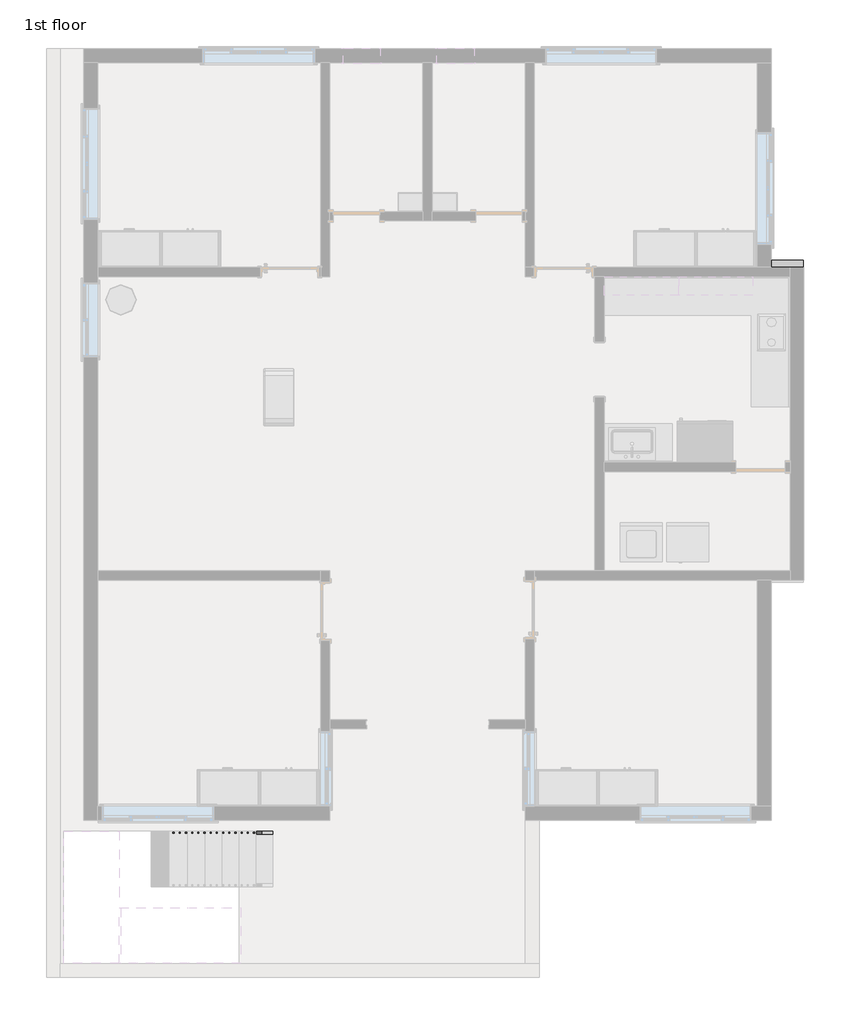
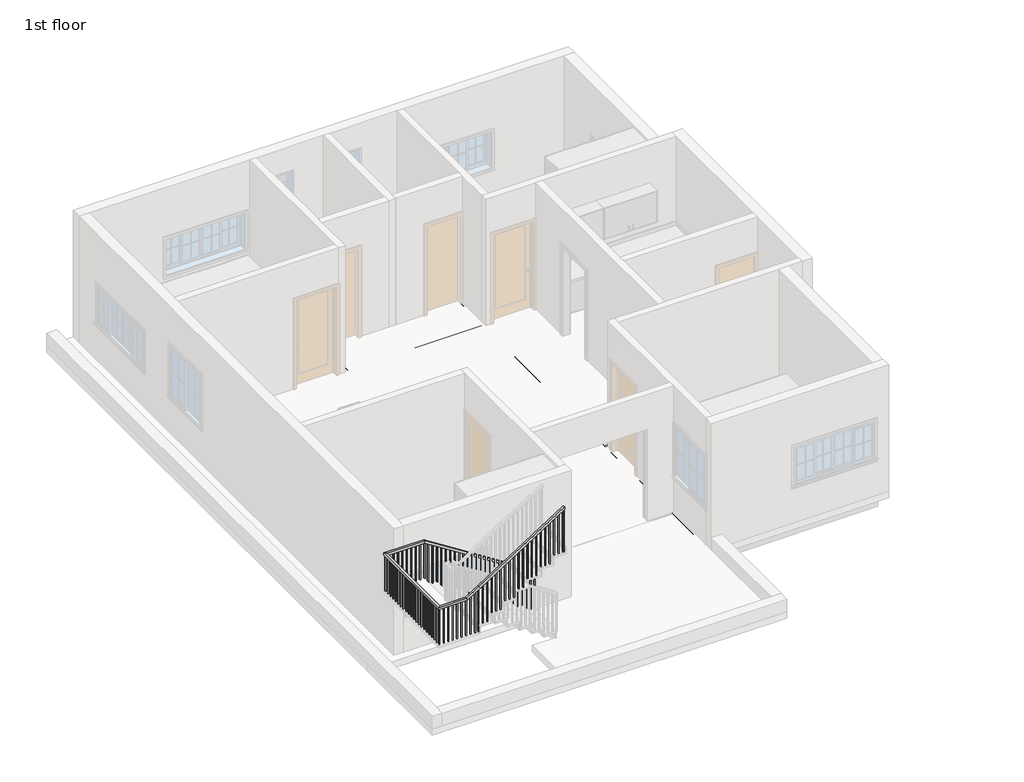
# One storey, part 2 of 4: 6 beams, 1 railing.
"""IFC4 building model written with IfcOpenShell, lengths in millimetres."""

from ifc_helpers import new_model, si_unit, frame, origin, place, context, project, spatial, polyline, outline, extrude, faceted_brep, element, save

model = new_model("IFC4")

# Units and contexts
model_context = context("Model", 3, world=origin())
ifc_project = project(units=[si_unit("LENGTHUNIT", "METRE", prefix="MILLI")], contexts=[model_context])

# Site, building, storey
site = spatial("IfcSite", under=ifc_project)
building = spatial("IfcBuilding", under=site)
storey = spatial("IfcBuildingStorey", under=building, Name="1st floor", Elevation=3810.0)

# Beams
placement = place(None, origin())
element("IfcBeam", 1, ObjectType="Concrete-Rectangular Beam", at=placement, inside=storey, context=model_context, shape_type="Brep", body=[
    faceted_brep([(-12413.6124084, 10142.6961804, 3810.0), (-12413.6124084, 9914.0961804, 3810.0), (-8794.1124084, 9914.0961804, 3810.0), (-8565.5124084, 9914.0961804, 3810.0), (-7117.7124084, 9914.0961804, 3810.0), (-6889.1124084, 9914.0961804, 3810.0), (-5441.3124084, 9914.0961804, 3810.0), (-5212.7124084, 9914.0961804, 3810.0), (-1593.2124084, 9914.0961804, 3810.0), (-1593.2124084, 10142.6961804, 3810.0), (-5174.6124084, 10142.6961804, 3810.0), (-5174.6124084, 9952.1961804, 3810.0), (-5479.4124084, 9952.1961804, 3810.0), (-5479.4124084, 10142.6961804, 3810.0), (-8451.2124084, 10142.6961804, 3810.0), (-8451.2124084, 9952.1961804, 3810.0), (-8756.0124084, 9952.1961804, 3810.0), (-8756.0124084, 10142.6961804, 3810.0), (-12413.6124084, 9914.0961804, 3505.2), (-8794.1124084, 9914.0961804, 3505.2), (-8565.5124084, 9914.0961804, 3505.2), (-7117.7124084, 9914.0961804, 3505.2), (-6889.1124084, 9914.0961804, 3505.2), (-5441.3124084, 9914.0961804, 3505.2), (-5212.7124084, 9914.0961804, 3505.2), (-1593.2124084, 9914.0961804, 3505.2), (-12413.6124084, 10142.6961804, 3505.2), (-8756.0124084, 10142.6961804, 3505.2), (-8756.0124084, 9952.1961804, 3505.2), (-8451.2124084, 9952.1961804, 3505.2), (-8451.2124084, 10142.6961804, 3505.2), (-5479.4124084, 10142.6961804, 3505.2), (-5479.4124084, 9952.1961804, 3505.2), (-5174.6124084, 9952.1961804, 3505.2), (-5174.6124084, 10142.6961804, 3505.2), (-1593.2124084, 10142.6961804, 3505.2)], [[[0, 1, 2, 3, 4, 5, 6, 7, 8, 9, 10, 11, 12, 13, 14, 15, 16, 17]], [[1, 18, 19, 20, 21, 22, 23, 24, 25, 8, 7, 6, 5, 4, 3, 2]], [[18, 26, 27, 28, 29, 30, 31, 32, 33, 34, 35, 25, 24, 23, 22, 21, 20, 19]], [[26, 0, 17, 27]], [[1, 0, 26, 18]], [[9, 8, 25, 35]], [[29, 15, 14, 30]], [[15, 29, 28, 16]], [[16, 28, 27, 17]], [[9, 35, 34, 10]], [[33, 11, 10, 34]], [[11, 33, 32, 12]], [[12, 32, 31, 13]], [[30, 14, 13, 31]]]),
])
element("IfcBeam", 2, ObjectType="Concrete-Rectangular Beam", at=placement, inside=storey, context=model_context, shape_type="SweptSolid", body=[
    extrude(outline(polyline([(-1593.2124084, 9875.9961804), (-1364.6124084, 9875.9961804), (-1364.6124084, 6751.7961804), (-1593.2124084, 6751.7961804), (-1593.2124084, 9875.9961804)])), frame((0.0, 0.0, 3505.2), z_axis=(0.0, 0.0, 1.0), x_axis=(1.0, 0.0, 0.0)), (0.0, 0.0, 1.0), 304.8),
])
element("IfcBeam", 3, ObjectType="Concrete-Rectangular Beam", at=placement, inside=storey, context=model_context, shape_type="Brep", body=[
    faceted_brep([(-843.9124084, 6713.6961804, 3810.0), (-843.9124084, 6485.0961804, 3810.0), (-843.9124084, 6485.0961804, 3505.2), (-843.9124084, 6713.6961804, 3505.2), (-1364.6124084, 6713.6961804, 3810.0), (-1364.6124084, 6485.0961804, 3810.0), (-1364.6124084, 6485.0961804, 3505.2), (-1364.6124084, 6713.6961804, 3505.2)], [[[0, 1, 2, 3]], [[1, 0, 4, 5]], [[2, 1, 5, 6]], [[3, 2, 6, 7]], [[0, 3, 7, 4]], [[5, 4, 7, 6]]]),
    faceted_brep([(-12413.6124084, 6485.0961804, 3810.0), (-12413.6124084, 6713.6961804, 3810.0), (-12413.6124084, 6713.6961804, 3505.2), (-12413.6124084, 6485.0961804, 3505.2), (-8756.0124084, 6713.6961804, 3810.0), (-8756.0124084, 6485.0961804, 3810.0), (-8756.0124084, 6485.0961804, 3505.2), (-8756.0124084, 6713.6961804, 3505.2), (-8794.1124084, 6485.0961804, 3810.0), (-8794.1124084, 6713.6961804, 3810.0), (-8794.1124084, 6485.0961804, 3505.2), (-8794.1124084, 6713.6961804, 3505.2)], [[[0, 1, 2, 3]], [[4, 5, 6, 7]], [[1, 0, 8, 5, 4, 9]], [[0, 3, 10, 6, 5, 8]], [[3, 2, 11, 7, 6, 10]], [[2, 1, 9, 4, 7, 11]]]),
    faceted_brep([(-1593.2124084, 6713.6961804, 3810.0), (-1593.2124084, 6485.0961804, 3810.0), (-1593.2124084, 6485.0961804, 3505.2), (-1593.2124084, 6713.6961804, 3505.2), (-5212.7124084, 6713.6961804, 3810.0), (-5250.8124084, 6713.6961804, 3810.0), (-5250.8124084, 6485.0961804, 3810.0), (-5212.7124084, 6485.0961804, 3810.0), (-5250.8124084, 6485.0961804, 3505.2), (-5212.7124084, 6485.0961804, 3505.2), (-5250.8124084, 6713.6961804, 3505.2), (-5212.7124084, 6713.6961804, 3505.2)], [[[0, 1, 2, 3]], [[1, 0, 4, 5, 6, 7]], [[2, 1, 7, 6, 8, 9]], [[3, 2, 9, 8, 10, 11]], [[0, 3, 11, 10, 5, 4]], [[6, 5, 10, 8]]]),
    faceted_brep([(-8527.4124084, 6485.0961804, 3810.0), (-8527.4124084, 6713.6961804, 3810.0), (-8527.4124084, 6713.6961804, 3505.2), (-8527.4124084, 6485.0961804, 3505.2), (-5479.4124084, 6713.6961804, 3810.0), (-5479.4124084, 6485.0961804, 3810.0), (-5479.4124084, 6485.0961804, 3505.2), (-5479.4124084, 6713.6961804, 3505.2)], [[[0, 1, 2, 3]], [[4, 5, 6, 7]], [[1, 0, 5, 4]], [[0, 3, 6, 5]], [[3, 2, 7, 6]], [[2, 1, 4, 7]]]),
])
element("IfcBeam", 4, ObjectType="Concrete-Rectangular Beam", at=placement, inside=storey, context=model_context, shape_type="Brep", body=[
    faceted_brep([(-5212.7124084, 9914.0961804, 3810.0), (-5441.3124084, 9914.0961804, 3810.0), (-5441.3124084, 7551.8961804, 3810.0), (-5441.3124084, 7323.2961804, 3810.0), (-5441.3124084, 6751.7961804, 3810.0), (-5250.8124084, 6751.7961804, 3810.0), (-5250.8124084, 6713.6961804, 3810.0), (-5212.7124084, 6713.6961804, 3810.0), (-5212.7124084, 9914.0961804, 3505.2), (-5212.7124084, 6713.6961804, 3505.2), (-5441.3124084, 9914.0961804, 3505.2), (-5250.8124084, 6713.6961804, 3505.2), (-5250.8124084, 6751.7961804, 3505.2), (-5441.3124084, 6751.7961804, 3505.2), (-5441.3124084, 7323.2961804, 3505.2), (-5441.3124084, 7551.8961804, 3505.2)], [[[0, 1, 2, 3, 4, 5, 6, 7]], [[8, 0, 7, 9]], [[10, 8, 9, 11, 12, 13, 14, 15]], [[1, 10, 15, 14, 13, 4, 3, 2]], [[1, 0, 8, 10]], [[9, 7, 6, 11]], [[12, 5, 4, 13]], [[5, 12, 11, 6]]]),
    faceted_brep([(-5212.7124084, -2201.7038196, 3810.0), (-5441.3124084, -2201.7038196, 3810.0), (-5441.3124084, -2201.7038196, 3505.2), (-5212.7124084, -2201.7038196, 3505.2), (-5441.3124084, 1430.4961804, 3505.2), (-5441.3124084, 1430.4961804, 3810.0), (-5212.7124084, 1430.4961804, 3810.0), (-5212.7124084, 1430.4961804, 3505.2), (-5441.3124084, -779.3038196, 3505.2), (-5441.3124084, -1007.9038196, 3505.2), (-5441.3124084, -1007.9038196, 3810.0), (-5441.3124084, -779.3038196, 3810.0)], [[[0, 1, 2, 3]], [[4, 5, 6, 7]], [[5, 4, 8, 9, 2, 1, 10, 11]], [[1, 0, 6, 5, 11, 10]], [[0, 3, 7, 6]], [[3, 2, 9, 8, 4, 7]]]),
    faceted_brep([(-5212.7124084, 6485.0961804, 3810.0), (-5212.7124084, 6485.0961804, 3505.2), (-5250.8124084, 6485.0961804, 3505.2), (-5250.8124084, 6485.0961804, 3810.0), (-5250.8124084, 6446.9961804, 3810.0), (-5441.3124084, 6446.9961804, 3810.0), (-5441.3124084, 1659.0961804, 3810.0), (-5403.2124084, 1659.0961804, 3810.0), (-5403.2124084, 1697.1961804, 3810.0), (-5212.7124084, 1697.1961804, 3810.0), (-5212.7124084, 1697.1961804, 3505.2), (-5403.2124084, 1697.1961804, 3505.2), (-5403.2124084, 1659.0961804, 3505.2), (-5441.3124084, 1659.0961804, 3505.2), (-5441.3124084, 6446.9961804, 3505.2), (-5250.8124084, 6446.9961804, 3505.2)], [[[0, 1, 2, 3]], [[0, 3, 4, 5, 6, 7, 8, 9]], [[1, 0, 9, 10]], [[2, 1, 10, 11, 12, 13, 14, 15]], [[6, 13, 12, 7]], [[13, 6, 5, 14]], [[15, 4, 3, 2]], [[4, 15, 14, 5]], [[8, 11, 10, 9]], [[11, 8, 7, 12]]]),
])
element("IfcBeam", 5, ObjectType="Concrete-Rectangular Beam", at=placement, inside=storey, context=model_context, shape_type="SweptSolid", body=[
    extrude(outline(polyline([(-7117.7124084, 9914.0961804), (-6889.1124084, 9914.0961804), (-6889.1124084, 7551.8961804), (-7117.7124084, 7551.8961804), (-7117.7124084, 9914.0961804)])), frame((0.0, 0.0, 3505.2), z_axis=(0.0, 0.0, 1.0), x_axis=(1.0, 0.0, 0.0)), (0.0, 0.0, 1.0), 304.8),
])
element("IfcBeam", 6, ObjectType="Concrete-Rectangular Beam", at=placement, inside=storey, context=model_context, shape_type="Brep", body=[
    faceted_brep([(-5441.3124084, 7323.2961804, 3810.0), (-5441.3124084, 7551.8961804, 3810.0), (-6889.1124084, 7551.8961804, 3810.0), (-7117.7124084, 7551.8961804, 3810.0), (-8565.5124084, 7551.8961804, 3810.0), (-8565.5124084, 7323.2961804, 3810.0), (-5441.3124084, 7323.2961804, 3505.2), (-8565.5124084, 7323.2961804, 3505.2), (-5441.3124084, 7551.8961804, 3505.2), (-8565.5124084, 7551.8961804, 3505.2), (-7117.7124084, 7551.8961804, 3505.2), (-6889.1124084, 7551.8961804, 3505.2)], [[[0, 1, 2, 3, 4, 5]], [[6, 0, 5, 7]], [[8, 6, 7, 9, 10, 11]], [[1, 8, 11, 10, 9, 4, 3, 2]], [[1, 0, 6, 8]], [[5, 4, 9, 7]]]),
])

# Railing
element("IfcRailing", 7, ObjectType="Handrail - Rectangular", at=placement, inside=storey, context=model_context, shape_type="SolidModel", body=[
    faceted_brep([(-9543.8120641, -2698.7669819, 4902.2), (-9543.8120641, -2698.7669819, 4841.986276), (-9543.8120641, -2647.9669819, 4841.986276), (-9543.8120641, -2647.9669819, 4902.2), (-12058.4120641, -2698.7669819, 6502.4), (-12073.205059, -2698.7669819, 6451.6), (-12073.205059, -2647.9669819, 6451.6), (-12058.4120641, -2647.9669819, 6502.4), (-12922.0120641, -2698.7669819, 6502.4), (-12922.0120641, -2698.7669819, 6451.6), (-12972.8120641, -2647.9669819, 6451.6), (-12972.8120641, -2647.9669819, 6502.4), (-12922.0120641, -4767.1038196, 6502.4), (-12922.0120641, -4767.1038196, 6451.6), (-12972.8120641, -4817.9038196, 6451.6), (-12972.8120641, -4817.9038196, 6502.4), (-12337.8120641, -4767.1038196, 6502.4), (-12323.0190691, -4767.1038196, 6451.6), (-12323.0190691, -4817.9038196, 6451.6), (-12337.8120641, -4817.9038196, 6502.4), (-12058.4120641, -4767.1038196, 6680.2), (-12031.138789, -4767.1038196, 6637.3419964), (-12031.138789, -4817.9038196, 6637.3419964), (-12058.4120641, -4817.9038196, 6680.2), (-10102.6120641, -4767.1038196, 7924.8), (-10102.6120641, -4817.9038196, 7924.8), (-10102.6120641, -4817.9038196, 7864.586276), (-10102.6120641, -4767.1038196, 7864.586276)], [[[0, 1, 2, 3]], [[1, 0, 4, 5]], [[2, 1, 5, 6]], [[3, 2, 6, 7]], [[0, 3, 7, 4]], [[5, 4, 8, 9]], [[6, 5, 9, 10]], [[7, 6, 10, 11]], [[4, 7, 11, 8]], [[9, 8, 12, 13]], [[10, 9, 13, 14]], [[11, 10, 14, 15]], [[8, 11, 15, 12]], [[13, 12, 16, 17]], [[14, 13, 17, 18]], [[15, 14, 18, 19]], [[12, 15, 19, 16]], [[17, 16, 20, 21]], [[18, 17, 21, 22]], [[19, 18, 22, 23]], [[16, 19, 23, 20]], [[24, 25, 26, 27]], [[21, 20, 24, 27]], [[22, 21, 27, 26]], [[23, 22, 26, 25]], [[20, 23, 25, 24]]]),
    extrude(outline(polyline([(7854.4840032, -10118.4870641), (7842.361276, -10137.5370641), (6832.6, -10137.5370641), (6832.6, -10118.4870641), (7854.4840032, -10118.4870641)])), frame((0.0, -4802.0288196, 0.0), z_axis=(0.0, 1.0, 0.0), x_axis=(0.0, 0.0, 1.0)), (0.0, 0.0, 1.0), 19.05),
    extrude(outline(polyline([(7789.8294578, -10220.0870641), (7777.7067305, -10239.1370641), (6832.6, -10239.1370641), (6832.6, -10220.0870641), (7789.8294578, -10220.0870641)])), frame((0.0, -4802.0288196, 0.0), z_axis=(0.0, 1.0, 0.0), x_axis=(0.0, 0.0, 1.0)), (0.0, 0.0, 1.0), 19.05),
    extrude(outline(polyline([(7725.1749123, -10321.6870641), (7713.0521851, -10340.7370641), (6832.6, -10340.7370641), (6832.6, -10321.6870641), (7725.1749123, -10321.6870641)])), frame((0.0, -4802.0288196, 0.0), z_axis=(0.0, 1.0, 0.0), x_axis=(0.0, 0.0, 1.0)), (0.0, 0.0, 1.0), 19.05),
    extrude(outline(polyline([(7660.5203669, -10423.2870641), (7648.3976396, -10442.3370641), (6654.8, -10442.3370641), (6654.8, -10423.2870641), (7660.5203669, -10423.2870641)])), frame((0.0, -4802.0288196, 0.0), z_axis=(0.0, 1.0, 0.0), x_axis=(0.0, 0.0, 1.0)), (0.0, 0.0, 1.0), 19.05),
    extrude(outline(polyline([(7595.8658214, -10524.8870641), (7583.7430941, -10543.9370641), (6654.8, -10543.9370641), (6654.8, -10524.8870641), (7595.8658214, -10524.8870641)])), frame((0.0, -4802.0288196, 0.0), z_axis=(0.0, 1.0, 0.0), x_axis=(0.0, 0.0, 1.0)), (0.0, 0.0, 1.0), 19.05),
    extrude(outline(polyline([(7531.211276, -10626.4870641), (7519.0885487, -10645.5370641), (6654.8, -10645.5370641), (6654.8, -10626.4870641), (7531.211276, -10626.4870641)])), frame((0.0, -4802.0288196, 0.0), z_axis=(0.0, 1.0, 0.0), x_axis=(0.0, 0.0, 1.0)), (0.0, 0.0, 1.0), 19.05),
    extrude(outline(polyline([(7466.5567305, -10728.0870641), (7454.4340032, -10747.1370641), (6477.0, -10747.1370641), (6477.0, -10728.0870641), (7466.5567305, -10728.0870641)])), frame((0.0, -4802.0288196, 0.0), z_axis=(0.0, 1.0, 0.0), x_axis=(0.0, 0.0, 1.0)), (0.0, 0.0, 1.0), 19.05),
    extrude(outline(polyline([(7401.9021851, -10829.6870641), (7389.7794578, -10848.7370641), (6477.0, -10848.7370641), (6477.0, -10829.6870641), (7401.9021851, -10829.6870641)])), frame((0.0, -4802.0288196, 0.0), z_axis=(0.0, 1.0, 0.0), x_axis=(0.0, 0.0, 1.0)), (0.0, 0.0, 1.0), 19.05),
    extrude(outline(polyline([(7337.2476396, -10931.2870641), (7325.1249123, -10950.3370641), (6477.0, -10950.3370641), (6477.0, -10931.2870641), (7337.2476396, -10931.2870641)])), frame((0.0, -4802.0288196, 0.0), z_axis=(0.0, 1.0, 0.0), x_axis=(0.0, 0.0, 1.0)), (0.0, 0.0, 1.0), 19.05),
    extrude(outline(polyline([(7272.5930941, -11032.8870641), (7260.4703669, -11051.9370641), (6299.2, -11051.9370641), (6299.2, -11032.8870641), (7272.5930941, -11032.8870641)])), frame((0.0, -4802.0288196, 0.0), z_axis=(0.0, 1.0, 0.0), x_axis=(0.0, 0.0, 1.0)), (0.0, 0.0, 1.0), 19.05),
    extrude(outline(polyline([(7207.9385487, -11134.4870641), (7195.8158214, -11153.5370641), (6299.2, -11153.5370641), (6299.2, -11134.4870641), (7207.9385487, -11134.4870641)])), frame((0.0, -4802.0288196, 0.0), z_axis=(0.0, 1.0, 0.0), x_axis=(0.0, 0.0, 1.0)), (0.0, 0.0, 1.0), 19.05),
    extrude(outline(polyline([(7143.2840032, -11236.0870641), (7131.161276, -11255.1370641), (6121.4, -11255.1370641), (6121.4, -11236.0870641), (7143.2840032, -11236.0870641)])), frame((0.0, -4802.0288196, 0.0), z_axis=(0.0, 1.0, 0.0), x_axis=(0.0, 0.0, 1.0)), (0.0, 0.0, 1.0), 19.05),
    extrude(outline(polyline([(7078.6294578, -11337.6870641), (7066.5067305, -11356.7370641), (6121.4, -11356.7370641), (6121.4, -11337.6870641), (7078.6294578, -11337.6870641)])), frame((0.0, -4802.0288196, 0.0), z_axis=(0.0, 1.0, 0.0), x_axis=(0.0, 0.0, 1.0)), (0.0, 0.0, 1.0), 19.05),
    extrude(outline(polyline([(7013.9749123, -11439.2870641), (7001.8521851, -11458.3370641), (6121.4, -11458.3370641), (6121.4, -11439.2870641), (7013.9749123, -11439.2870641)])), frame((0.0, -4802.0288196, 0.0), z_axis=(0.0, 1.0, 0.0), x_axis=(0.0, 0.0, 1.0)), (0.0, 0.0, 1.0), 19.05),
    extrude(outline(polyline([(6949.3203669, -11540.8870641), (6937.1976396, -11559.9370641), (5943.6, -11559.9370641), (5943.6, -11540.8870641), (6949.3203669, -11540.8870641)])), frame((0.0, -4802.0288196, 0.0), z_axis=(0.0, 1.0, 0.0), x_axis=(0.0, 0.0, 1.0)), (0.0, 0.0, 1.0), 19.05),
    extrude(outline(polyline([(6884.6658214, -11642.4870641), (6872.5430941, -11661.5370641), (5943.6, -11661.5370641), (5943.6, -11642.4870641), (6884.6658214, -11642.4870641)])), frame((0.0, -4802.0288196, 0.0), z_axis=(0.0, 1.0, 0.0), x_axis=(0.0, 0.0, 1.0)), (0.0, 0.0, 1.0), 19.05),
    extrude(outline(polyline([(6820.011276, -11744.0870641), (6807.8885487, -11763.1370641), (5943.6, -11763.1370641), (5943.6, -11744.0870641), (6820.011276, -11744.0870641)])), frame((0.0, -4802.0288196, 0.0), z_axis=(0.0, 1.0, 0.0), x_axis=(0.0, 0.0, 1.0)), (0.0, 0.0, 1.0), 19.05),
    extrude(outline(polyline([(6755.3567305, -11845.6870641), (6743.2340032, -11864.7370641), (5765.8, -11864.7370641), (5765.8, -11845.6870641), (6755.3567305, -11845.6870641)])), frame((0.0, -4802.0288196, 0.0), z_axis=(0.0, 1.0, 0.0), x_axis=(0.0, 0.0, 1.0)), (0.0, 0.0, 1.0), 19.05),
    extrude(outline(polyline([(6690.7021851, -11947.2870641), (6678.5794578, -11966.3370641), (5765.8, -11966.3370641), (5765.8, -11947.2870641), (6690.7021851, -11947.2870641)])), frame((0.0, -4802.0288196, 0.0), z_axis=(0.0, 1.0, 0.0), x_axis=(0.0, 0.0, 1.0)), (0.0, 0.0, 1.0), 19.05),
    extrude(outline(polyline([(6577.5567305, -12125.0870641), (6565.4340032, -12144.1370641), (5588.0, -12144.1370641), (5588.0, -12125.0870641), (6577.5567305, -12125.0870641)])), frame((0.0, -4802.0288196, 0.0), z_axis=(0.0, 1.0, 0.0), x_axis=(0.0, 0.0, 1.0)), (0.0, 0.0, 1.0), 19.05),
    extrude(outline(polyline([(6512.9021851, -12226.6870641), (6500.7794578, -12245.7370641), (5588.0, -12245.7370641), (5588.0, -12226.6870641), (6512.9021851, -12226.6870641)])), frame((0.0, -4802.0288196, 0.0), z_axis=(0.0, 1.0, 0.0), x_axis=(0.0, 0.0, 1.0)), (0.0, 0.0, 1.0), 19.05),
    extrude(outline(polyline([(-12347.3370641, -4802.0288196), (-12347.3370641, -4782.9788196), (-12328.2870641, -4782.9788196), (-12328.2870641, -4802.0288196), (-12347.3370641, -4802.0288196)])), frame((0.0, 0.0, 5588.0), z_axis=(0.0, 0.0, 1.0), x_axis=(1.0, 0.0, 0.0)), (0.0, 0.0, 1.0), 863.6),
    extrude(outline(polyline([(-12448.9370641, -4802.0288196), (-12448.9370641, -4782.9788196), (-12429.8870641, -4782.9788196), (-12429.8870641, -4802.0288196), (-12448.9370641, -4802.0288196)])), frame((0.0, 0.0, 5588.0), z_axis=(0.0, 0.0, 1.0), x_axis=(1.0, 0.0, 0.0)), (0.0, 0.0, 1.0), 863.6),
    extrude(outline(polyline([(-12550.5370641, -4802.0288196), (-12550.5370641, -4782.9788196), (-12531.4870641, -4782.9788196), (-12531.4870641, -4802.0288196), (-12550.5370641, -4802.0288196)])), frame((0.0, 0.0, 5588.0), z_axis=(0.0, 0.0, 1.0), x_axis=(1.0, 0.0, 0.0)), (0.0, 0.0, 1.0), 863.6),
    extrude(outline(polyline([(-12652.1370641, -4802.0288196), (-12652.1370641, -4782.9788196), (-12633.0870641, -4782.9788196), (-12633.0870641, -4802.0288196), (-12652.1370641, -4802.0288196)])), frame((0.0, 0.0, 5588.0), z_axis=(0.0, 0.0, 1.0), x_axis=(1.0, 0.0, 0.0)), (0.0, 0.0, 1.0), 863.6),
    extrude(outline(polyline([(-12753.7370641, -4802.0288196), (-12753.7370641, -4782.9788196), (-12734.6870641, -4782.9788196), (-12734.6870641, -4802.0288196), (-12753.7370641, -4802.0288196)])), frame((0.0, 0.0, 5588.0), z_axis=(0.0, 0.0, 1.0), x_axis=(1.0, 0.0, 0.0)), (0.0, 0.0, 1.0), 863.6),
    extrude(outline(polyline([(-12855.3370641, -4802.0288196), (-12855.3370641, -4782.9788196), (-12836.2870641, -4782.9788196), (-12836.2870641, -4802.0288196), (-12855.3370641, -4802.0288196)])), frame((0.0, 0.0, 5588.0), z_axis=(0.0, 0.0, 1.0), x_axis=(1.0, 0.0, 0.0)), (0.0, 0.0, 1.0), 863.6),
    extrude(outline(polyline([(-12956.9370641, -4695.8419819), (-12937.8870641, -4695.8419819), (-12937.8870641, -4714.8919819), (-12956.9370641, -4714.8919819), (-12956.9370641, -4695.8419819)])), frame((0.0, 0.0, 5588.0), z_axis=(0.0, 0.0, 1.0), x_axis=(1.0, 0.0, 0.0)), (0.0, 0.0, 1.0), 863.6),
    extrude(outline(polyline([(-12956.9370641, -4594.2419819), (-12937.8870641, -4594.2419819), (-12937.8870641, -4613.2919819), (-12956.9370641, -4613.2919819), (-12956.9370641, -4594.2419819)])), frame((0.0, 0.0, 5588.0), z_axis=(0.0, 0.0, 1.0), x_axis=(1.0, 0.0, 0.0)), (0.0, 0.0, 1.0), 863.6),
    extrude(outline(polyline([(-12956.9370641, -4492.6419819), (-12937.8870641, -4492.6419819), (-12937.8870641, -4511.6919819), (-12956.9370641, -4511.6919819), (-12956.9370641, -4492.6419819)])), frame((0.0, 0.0, 5588.0), z_axis=(0.0, 0.0, 1.0), x_axis=(1.0, 0.0, 0.0)), (0.0, 0.0, 1.0), 863.6),
    extrude(outline(polyline([(-12956.9370641, -4391.0419819), (-12937.8870641, -4391.0419819), (-12937.8870641, -4410.0919819), (-12956.9370641, -4410.0919819), (-12956.9370641, -4391.0419819)])), frame((0.0, 0.0, 5588.0), z_axis=(0.0, 0.0, 1.0), x_axis=(1.0, 0.0, 0.0)), (0.0, 0.0, 1.0), 863.6),
    extrude(outline(polyline([(-12956.9370641, -4289.4419819), (-12937.8870641, -4289.4419819), (-12937.8870641, -4308.4919819), (-12956.9370641, -4308.4919819), (-12956.9370641, -4289.4419819)])), frame((0.0, 0.0, 5588.0), z_axis=(0.0, 0.0, 1.0), x_axis=(1.0, 0.0, 0.0)), (0.0, 0.0, 1.0), 863.6),
    extrude(outline(polyline([(-12956.9370641, -4187.8419819), (-12937.8870641, -4187.8419819), (-12937.8870641, -4206.8919819), (-12956.9370641, -4206.8919819), (-12956.9370641, -4187.8419819)])), frame((0.0, 0.0, 5588.0), z_axis=(0.0, 0.0, 1.0), x_axis=(1.0, 0.0, 0.0)), (0.0, 0.0, 1.0), 863.6),
    extrude(outline(polyline([(-12956.9370641, -4086.2419819), (-12937.8870641, -4086.2419819), (-12937.8870641, -4105.2919819), (-12956.9370641, -4105.2919819), (-12956.9370641, -4086.2419819)])), frame((0.0, 0.0, 5588.0), z_axis=(0.0, 0.0, 1.0), x_axis=(1.0, 0.0, 0.0)), (0.0, 0.0, 1.0), 863.6),
    extrude(outline(polyline([(-12956.9370641, -3984.6419819), (-12937.8870641, -3984.6419819), (-12937.8870641, -4003.6919819), (-12956.9370641, -4003.6919819), (-12956.9370641, -3984.6419819)])), frame((0.0, 0.0, 5588.0), z_axis=(0.0, 0.0, 1.0), x_axis=(1.0, 0.0, 0.0)), (0.0, 0.0, 1.0), 863.6),
    extrude(outline(polyline([(-12956.9370641, -3883.0419819), (-12937.8870641, -3883.0419819), (-12937.8870641, -3902.0919819), (-12956.9370641, -3902.0919819), (-12956.9370641, -3883.0419819)])), frame((0.0, 0.0, 5588.0), z_axis=(0.0, 0.0, 1.0), x_axis=(1.0, 0.0, 0.0)), (0.0, 0.0, 1.0), 863.6),
    extrude(outline(polyline([(-12956.9370641, -3781.4419819), (-12937.8870641, -3781.4419819), (-12937.8870641, -3800.4919819), (-12956.9370641, -3800.4919819), (-12956.9370641, -3781.4419819)])), frame((0.0, 0.0, 5588.0), z_axis=(0.0, 0.0, 1.0), x_axis=(1.0, 0.0, 0.0)), (0.0, 0.0, 1.0), 863.6),
    extrude(outline(polyline([(-12956.9370641, -3679.8419819), (-12937.8870641, -3679.8419819), (-12937.8870641, -3698.8919819), (-12956.9370641, -3698.8919819), (-12956.9370641, -3679.8419819)])), frame((0.0, 0.0, 5588.0), z_axis=(0.0, 0.0, 1.0), x_axis=(1.0, 0.0, 0.0)), (0.0, 0.0, 1.0), 863.6),
    extrude(outline(polyline([(-12956.9370641, -3578.2419819), (-12937.8870641, -3578.2419819), (-12937.8870641, -3597.2919819), (-12956.9370641, -3597.2919819), (-12956.9370641, -3578.2419819)])), frame((0.0, 0.0, 5588.0), z_axis=(0.0, 0.0, 1.0), x_axis=(1.0, 0.0, 0.0)), (0.0, 0.0, 1.0), 863.6),
    extrude(outline(polyline([(-12956.9370641, -3476.6419819), (-12937.8870641, -3476.6419819), (-12937.8870641, -3495.6919819), (-12956.9370641, -3495.6919819), (-12956.9370641, -3476.6419819)])), frame((0.0, 0.0, 5588.0), z_axis=(0.0, 0.0, 1.0), x_axis=(1.0, 0.0, 0.0)), (0.0, 0.0, 1.0), 863.6),
    extrude(outline(polyline([(-12956.9370641, -3375.0419819), (-12937.8870641, -3375.0419819), (-12937.8870641, -3394.0919819), (-12956.9370641, -3394.0919819), (-12956.9370641, -3375.0419819)])), frame((0.0, 0.0, 5588.0), z_axis=(0.0, 0.0, 1.0), x_axis=(1.0, 0.0, 0.0)), (0.0, 0.0, 1.0), 863.6),
    extrude(outline(polyline([(-12956.9370641, -3273.4419819), (-12937.8870641, -3273.4419819), (-12937.8870641, -3292.4919819), (-12956.9370641, -3292.4919819), (-12956.9370641, -3273.4419819)])), frame((0.0, 0.0, 5588.0), z_axis=(0.0, 0.0, 1.0), x_axis=(1.0, 0.0, 0.0)), (0.0, 0.0, 1.0), 863.6),
    extrude(outline(polyline([(-12956.9370641, -3171.8419819), (-12937.8870641, -3171.8419819), (-12937.8870641, -3190.8919819), (-12956.9370641, -3190.8919819), (-12956.9370641, -3171.8419819)])), frame((0.0, 0.0, 5588.0), z_axis=(0.0, 0.0, 1.0), x_axis=(1.0, 0.0, 0.0)), (0.0, 0.0, 1.0), 863.6),
    extrude(outline(polyline([(-12956.9370641, -3070.2419819), (-12937.8870641, -3070.2419819), (-12937.8870641, -3089.2919819), (-12956.9370641, -3089.2919819), (-12956.9370641, -3070.2419819)])), frame((0.0, 0.0, 5588.0), z_axis=(0.0, 0.0, 1.0), x_axis=(1.0, 0.0, 0.0)), (0.0, 0.0, 1.0), 863.6),
    extrude(outline(polyline([(-12956.9370641, -2968.6419819), (-12937.8870641, -2968.6419819), (-12937.8870641, -2987.6919819), (-12956.9370641, -2987.6919819), (-12956.9370641, -2968.6419819)])), frame((0.0, 0.0, 5588.0), z_axis=(0.0, 0.0, 1.0), x_axis=(1.0, 0.0, 0.0)), (0.0, 0.0, 1.0), 863.6),
    extrude(outline(polyline([(-12956.9370641, -2867.0419819), (-12937.8870641, -2867.0419819), (-12937.8870641, -2886.0919819), (-12956.9370641, -2886.0919819), (-12956.9370641, -2867.0419819)])), frame((0.0, 0.0, 5588.0), z_axis=(0.0, 0.0, 1.0), x_axis=(1.0, 0.0, 0.0)), (0.0, 0.0, 1.0), 863.6),
    extrude(outline(polyline([(-12956.9370641, -2765.4419819), (-12937.8870641, -2765.4419819), (-12937.8870641, -2784.4919819), (-12956.9370641, -2784.4919819), (-12956.9370641, -2765.4419819)])), frame((0.0, 0.0, 5588.0), z_axis=(0.0, 0.0, 1.0), x_axis=(1.0, 0.0, 0.0)), (0.0, 0.0, 1.0), 863.6),
    extrude(outline(polyline([(-12861.6870641, -2663.8419819), (-12861.6870641, -2682.8919819), (-12880.7370641, -2682.8919819), (-12880.7370641, -2663.8419819), (-12861.6870641, -2663.8419819)])), frame((0.0, 0.0, 5588.0), z_axis=(0.0, 0.0, 1.0), x_axis=(1.0, 0.0, 0.0)), (0.0, 0.0, 1.0), 863.6),
    extrude(outline(polyline([(-12760.0870641, -2663.8419819), (-12760.0870641, -2682.8919819), (-12779.1370641, -2682.8919819), (-12779.1370641, -2663.8419819), (-12760.0870641, -2663.8419819)])), frame((0.0, 0.0, 5588.0), z_axis=(0.0, 0.0, 1.0), x_axis=(1.0, 0.0, 0.0)), (0.0, 0.0, 1.0), 863.6),
    extrude(outline(polyline([(-12658.4870641, -2663.8419819), (-12658.4870641, -2682.8919819), (-12677.5370641, -2682.8919819), (-12677.5370641, -2663.8419819), (-12658.4870641, -2663.8419819)])), frame((0.0, 0.0, 5588.0), z_axis=(0.0, 0.0, 1.0), x_axis=(1.0, 0.0, 0.0)), (0.0, 0.0, 1.0), 863.6),
    extrude(outline(polyline([(-12556.8870641, -2663.8419819), (-12556.8870641, -2682.8919819), (-12575.9370641, -2682.8919819), (-12575.9370641, -2663.8419819), (-12556.8870641, -2663.8419819)])), frame((0.0, 0.0, 5588.0), z_axis=(0.0, 0.0, 1.0), x_axis=(1.0, 0.0, 0.0)), (0.0, 0.0, 1.0), 863.6),
    extrude(outline(polyline([(-12455.2870641, -2663.8419819), (-12455.2870641, -2682.8919819), (-12474.3370641, -2682.8919819), (-12474.3370641, -2663.8419819), (-12455.2870641, -2663.8419819)])), frame((0.0, 0.0, 5588.0), z_axis=(0.0, 0.0, 1.0), x_axis=(1.0, 0.0, 0.0)), (0.0, 0.0, 1.0), 863.6),
    extrude(outline(polyline([(-12353.6870641, -2663.8419819), (-12353.6870641, -2682.8919819), (-12372.7370641, -2682.8919819), (-12372.7370641, -2663.8419819), (-12353.6870641, -2663.8419819)])), frame((0.0, 0.0, 5588.0), z_axis=(0.0, 0.0, 1.0), x_axis=(1.0, 0.0, 0.0)), (0.0, 0.0, 1.0), 863.6),
    extrude(outline(polyline([(-12252.0870641, -2663.8419819), (-12252.0870641, -2682.8919819), (-12271.1370641, -2682.8919819), (-12271.1370641, -2663.8419819), (-12252.0870641, -2663.8419819)])), frame((0.0, 0.0, 5588.0), z_axis=(0.0, 0.0, 1.0), x_axis=(1.0, 0.0, 0.0)), (0.0, 0.0, 1.0), 863.6),
    extrude(outline(polyline([(-12150.4870641, -2663.8419819), (-12150.4870641, -2682.8919819), (-12169.5370641, -2682.8919819), (-12169.5370641, -2663.8419819), (-12150.4870641, -2663.8419819)])), frame((0.0, 0.0, 5588.0), z_axis=(0.0, 0.0, 1.0), x_axis=(1.0, 0.0, 0.0)), (0.0, 0.0, 1.0), 863.6),
    extrude(outline(polyline([(6387.6340032, -11972.6870641), (6399.7567305, -11991.7370641), (5410.2, -11991.7370641), (5410.2, -11972.6870641), (6387.6340032, -11972.6870641)])), frame((0.0, -2682.8919819, 0.0), z_axis=(0.0, 1.0, 0.0), x_axis=(0.0, 0.0, 1.0)), (0.0, 0.0, 1.0), 19.05),
    extrude(outline(polyline([(6322.9794578, -11871.0870641), (6335.1021851, -11890.1370641), (5410.2, -11890.1370641), (5410.2, -11871.0870641), (6322.9794578, -11871.0870641)])), frame((0.0, -2682.8919819, 0.0), z_axis=(0.0, 1.0, 0.0), x_axis=(0.0, 0.0, 1.0)), (0.0, 0.0, 1.0), 19.05),
    extrude(outline(polyline([(6258.3249123, -11769.4870641), (6270.4476396, -11788.5370641), (5410.2, -11788.5370641), (5410.2, -11769.4870641), (6258.3249123, -11769.4870641)])), frame((0.0, -2682.8919819, 0.0), z_axis=(0.0, 1.0, 0.0), x_axis=(0.0, 0.0, 1.0)), (0.0, 0.0, 1.0), 19.05),
    extrude(outline(polyline([(6193.6703669, -11667.8870641), (6205.7930941, -11686.9370641), (5232.4, -11686.9370641), (5232.4, -11667.8870641), (6193.6703669, -11667.8870641)])), frame((0.0, -2682.8919819, 0.0), z_axis=(0.0, 1.0, 0.0), x_axis=(0.0, 0.0, 1.0)), (0.0, 0.0, 1.0), 19.05),
    extrude(outline(polyline([(6129.0158214, -11566.2870641), (6141.1385487, -11585.3370641), (5232.4, -11585.3370641), (5232.4, -11566.2870641), (6129.0158214, -11566.2870641)])), frame((0.0, -2682.8919819, 0.0), z_axis=(0.0, 1.0, 0.0), x_axis=(0.0, 0.0, 1.0)), (0.0, 0.0, 1.0), 19.05),
    extrude(outline(polyline([(6064.361276, -11464.6870641), (6076.4840032, -11483.7370641), (5054.6, -11483.7370641), (5054.6, -11464.6870641), (6064.361276, -11464.6870641)])), frame((0.0, -2682.8919819, 0.0), z_axis=(0.0, 1.0, 0.0), x_axis=(0.0, 0.0, 1.0)), (0.0, 0.0, 1.0), 19.05),
    extrude(outline(polyline([(5999.7067305, -11363.0870641), (6011.8294578, -11382.1370641), (5054.6, -11382.1370641), (5054.6, -11363.0870641), (5999.7067305, -11363.0870641)])), frame((0.0, -2682.8919819, 0.0), z_axis=(0.0, 1.0, 0.0), x_axis=(0.0, 0.0, 1.0)), (0.0, 0.0, 1.0), 19.05),
    extrude(outline(polyline([(5935.0521851, -11261.4870641), (5947.1749123, -11280.5370641), (5054.6, -11280.5370641), (5054.6, -11261.4870641), (5935.0521851, -11261.4870641)])), frame((0.0, -2682.8919819, 0.0), z_axis=(0.0, 1.0, 0.0), x_axis=(0.0, 0.0, 1.0)), (0.0, 0.0, 1.0), 19.05),
    extrude(outline(polyline([(5870.3976396, -11159.8870641), (5882.5203669, -11178.9370641), (4876.8, -11178.9370641), (4876.8, -11159.8870641), (5870.3976396, -11159.8870641)])), frame((0.0, -2682.8919819, 0.0), z_axis=(0.0, 1.0, 0.0), x_axis=(0.0, 0.0, 1.0)), (0.0, 0.0, 1.0), 19.05),
    extrude(outline(polyline([(5805.7430941, -11058.2870641), (5817.8658214, -11077.3370641), (4876.8, -11077.3370641), (4876.8, -11058.2870641), (5805.7430941, -11058.2870641)])), frame((0.0, -2682.8919819, 0.0), z_axis=(0.0, 1.0, 0.0), x_axis=(0.0, 0.0, 1.0)), (0.0, 0.0, 1.0), 19.05),
    extrude(outline(polyline([(5741.0885487, -10956.6870641), (5753.211276, -10975.7370641), (4876.8, -10975.7370641), (4876.8, -10956.6870641), (5741.0885487, -10956.6870641)])), frame((0.0, -2682.8919819, 0.0), z_axis=(0.0, 1.0, 0.0), x_axis=(0.0, 0.0, 1.0)), (0.0, 0.0, 1.0), 19.05),
    extrude(outline(polyline([(5676.4340032, -10855.0870641), (5688.5567305, -10874.1370641), (4699.0, -10874.1370641), (4699.0, -10855.0870641), (5676.4340032, -10855.0870641)])), frame((0.0, -2682.8919819, 0.0), z_axis=(0.0, 1.0, 0.0), x_axis=(0.0, 0.0, 1.0)), (0.0, 0.0, 1.0), 19.05),
    extrude(outline(polyline([(5611.7794578, -10753.4870641), (5623.9021851, -10772.5370641), (4699.0, -10772.5370641), (4699.0, -10753.4870641), (5611.7794578, -10753.4870641)])), frame((0.0, -2682.8919819, 0.0), z_axis=(0.0, 1.0, 0.0), x_axis=(0.0, 0.0, 1.0)), (0.0, 0.0, 1.0), 19.05),
    extrude(outline(polyline([(5547.1249123, -10651.8870641), (5559.2476396, -10670.9370641), (4699.0, -10670.9370641), (4699.0, -10651.8870641), (5547.1249123, -10651.8870641)])), frame((0.0, -2682.8919819, 0.0), z_axis=(0.0, 1.0, 0.0), x_axis=(0.0, 0.0, 1.0)), (0.0, 0.0, 1.0), 19.05),
    extrude(outline(polyline([(5482.4703669, -10550.2870641), (5494.5930941, -10569.3370641), (4521.2, -10569.3370641), (4521.2, -10550.2870641), (5482.4703669, -10550.2870641)])), frame((0.0, -2682.8919819, 0.0), z_axis=(0.0, 1.0, 0.0), x_axis=(0.0, 0.0, 1.0)), (0.0, 0.0, 1.0), 19.05),
    extrude(outline(polyline([(5417.8158214, -10448.6870641), (5429.9385487, -10467.7370641), (4521.2, -10467.7370641), (4521.2, -10448.6870641), (5417.8158214, -10448.6870641)])), frame((0.0, -2682.8919819, 0.0), z_axis=(0.0, 1.0, 0.0), x_axis=(0.0, 0.0, 1.0)), (0.0, 0.0, 1.0), 19.05),
    extrude(outline(polyline([(5353.161276, -10347.0870641), (5365.2840032, -10366.1370641), (4343.4, -10366.1370641), (4343.4, -10347.0870641), (5353.161276, -10347.0870641)])), frame((0.0, -2682.8919819, 0.0), z_axis=(0.0, 1.0, 0.0), x_axis=(0.0, 0.0, 1.0)), (0.0, 0.0, 1.0), 19.05),
    extrude(outline(polyline([(5288.5067305, -10245.4870641), (5300.6294578, -10264.5370641), (4343.4, -10264.5370641), (4343.4, -10245.4870641), (5288.5067305, -10245.4870641)])), frame((0.0, -2682.8919819, 0.0), z_axis=(0.0, 1.0, 0.0), x_axis=(0.0, 0.0, 1.0)), (0.0, 0.0, 1.0), 19.05),
    extrude(outline(polyline([(5223.8521851, -10143.8870641), (5235.9749123, -10162.9370641), (4343.4, -10162.9370641), (4343.4, -10143.8870641), (5223.8521851, -10143.8870641)])), frame((0.0, -2682.8919819, 0.0), z_axis=(0.0, 1.0, 0.0), x_axis=(0.0, 0.0, 1.0)), (0.0, 0.0, 1.0), 19.05),
    extrude(outline(polyline([(5159.1976396, -10042.2870641), (5171.3203669, -10061.3370641), (4165.6, -10061.3370641), (4165.6, -10042.2870641), (5159.1976396, -10042.2870641)])), frame((0.0, -2682.8919819, 0.0), z_axis=(0.0, 1.0, 0.0), x_axis=(0.0, 0.0, 1.0)), (0.0, 0.0, 1.0), 19.05),
    extrude(outline(polyline([(5094.5430941, -9940.6870641), (5106.6658214, -9959.7370641), (4165.6, -9959.7370641), (4165.6, -9940.6870641), (5094.5430941, -9940.6870641)])), frame((0.0, -2682.8919819, 0.0), z_axis=(0.0, 1.0, 0.0), x_axis=(0.0, 0.0, 1.0)), (0.0, 0.0, 1.0), 19.05),
    extrude(outline(polyline([(5029.8885487, -9839.0870641), (5042.011276, -9858.1370641), (4165.6, -9858.1370641), (4165.6, -9839.0870641), (5029.8885487, -9839.0870641)])), frame((0.0, -2682.8919819, 0.0), z_axis=(0.0, 1.0, 0.0), x_axis=(0.0, 0.0, 1.0)), (0.0, 0.0, 1.0), 19.05),
    extrude(outline(polyline([(4965.2340032, -9737.4870641), (4977.3567305, -9756.5370641), (3987.8, -9756.5370641), (3987.8, -9737.4870641), (4965.2340032, -9737.4870641)])), frame((0.0, -2682.8919819, 0.0), z_axis=(0.0, 1.0, 0.0), x_axis=(0.0, 0.0, 1.0)), (0.0, 0.0, 1.0), 19.05),
    extrude(outline(polyline([(4900.5794578, -9635.8870641), (4912.7021851, -9654.9370641), (3987.8, -9654.9370641), (3987.8, -9635.8870641), (4900.5794578, -9635.8870641)])), frame((0.0, -2682.8919819, 0.0), z_axis=(0.0, 1.0, 0.0), x_axis=(0.0, 0.0, 1.0)), (0.0, 0.0, 1.0), 19.05),
    extrude(outline(polyline([(6626.0476396, -12048.8870641), (6613.9249123, -12067.9370641), (5588.0, -12067.9370641), (5588.0, -12048.8870641), (6626.0476396, -12048.8870641)])), frame((0.0, -4802.0288196, 0.0), z_axis=(0.0, 1.0, 0.0), x_axis=(0.0, 0.0, 1.0)), (0.0, 0.0, 1.0), 19.05),
    extrude(outline(polyline([(-12956.9370641, -4782.9788196), (-12937.8870641, -4782.9788196), (-12937.8870641, -4802.0288196), (-12956.9370641, -4802.0288196), (-12956.9370641, -4782.9788196)])), frame((0.0, 0.0, 5588.0), z_axis=(0.0, 0.0, 1.0), x_axis=(1.0, 0.0, 0.0)), (0.0, 0.0, 1.0), 863.6),
    extrude(outline(polyline([(-12937.8870641, -2663.8419819), (-12937.8870641, -2682.8919819), (-12956.9370641, -2682.8919819), (-12956.9370641, -2663.8419819), (-12937.8870641, -2663.8419819)])), frame((0.0, 0.0, 5588.0), z_axis=(0.0, 0.0, 1.0), x_axis=(1.0, 0.0, 0.0)), (0.0, 0.0, 1.0), 863.6),
    extrude(outline(polyline([(6436.1249123, -12048.8870641), (6448.2476396, -12067.9370641), (5588.0, -12067.9370641), (5588.0, -12048.8870641), (6436.1249123, -12048.8870641)])), frame((0.0, -2682.8919819, 0.0), z_axis=(0.0, 1.0, 0.0), x_axis=(0.0, 0.0, 1.0)), (0.0, 0.0, 1.0), 19.05),
    extrude(outline(polyline([(7864.586276, -10102.6120641), (7852.4635487, -10121.6620641), (6832.6, -10121.6620641), (6832.6, -10102.6120641), (7864.586276, -10102.6120641)])), frame((0.0, -4802.0288196, 0.0), z_axis=(0.0, 1.0, 0.0), x_axis=(0.0, 0.0, 1.0)), (0.0, 0.0, 1.0), 19.05),
    extrude(outline(polyline([(4841.986276, -9543.8120641), (4854.1090032, -9562.8620641), (3987.8, -9562.8620641), (3987.8, -9543.8120641), (4841.986276, -9543.8120641)])), frame((0.0, -2682.8919819, 0.0), z_axis=(0.0, 1.0, 0.0), x_axis=(0.0, 0.0, 1.0)), (0.0, 0.0, 1.0), 19.05),
])

save(model, "model.ifc")

# Revit data of these elements
# Type "Concrete-Rectangular Beam"
#   Assembly Code = "B10"
#   Length [instance default] = 5' - 0"
#   b = 0' - 9"
#   h = 1' - 0"
#   Structural Material [instance default] = Concrete, Cast-in-Place gray
# Type "Handrail - Rectangular"
#   Assembly Code = "C2010400"
#   built-in parameter 1008612 = 0.0416667 (stored number, unit not read)
#   built-in parameter 1008611 = 0.0416667 (stored number, unit not read)
#   built-in parameter 1008609 = 0.333333 (stored number, unit not read)
#   built-in parameter 1008604 = 0.166667 (stored number, unit not read)
#   built-in parameter 1008603 = 0.166667 (stored number, unit not read)
#   Railing Height = 3' - 0"
#   built-in parameter 1008630 = 2
#   built-in parameter 1008610 = 2
#   built-in parameter 1008618 = Baluster - Square : 3/4"
# Elements 1, 2, 3, 4, 5, 6 (IfcBeam, "Concrete-Rectangular Beam")
#   Structural Material = Concrete, Cast-in-Place gray
#   Phase Created = New Construction
#   Materials on its faces: "Concrete, Cast-in-Place gray"
# Element 7 (IfcRailing, "Handrail - Rectangular")
#   Phase Created = New Construction
# Materials
#   "Concrete, Cast-in-Place gray": class "Concrete", colour RGB 192 192 192, transparency 0, Description = "Cast-in-place concrete", Cost = 0
